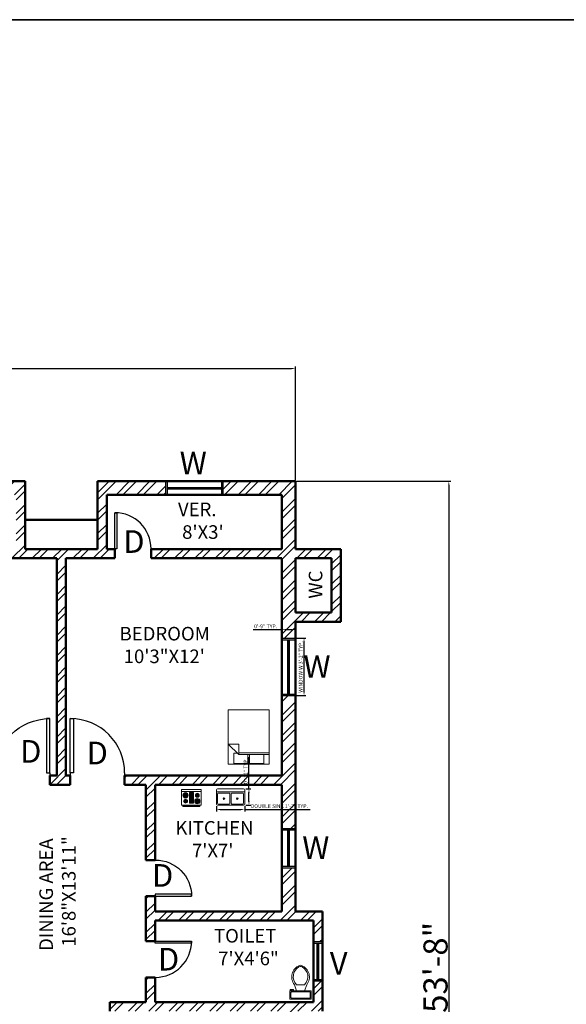
# Model space of a CAD drawing. Units: inches. Extents: x -31485 to -28799, y 18003 to 19130.
# Tile 10 of 15: x -30079 to -29717, y 18478 to 19130. Entities that reach past the tile are written whole.
import ezdxf

# ---------------------------------------------------------------- set-up
doc = ezdxf.new("R2010")
doc.units = ezdxf.units.IN
for name, color, linetype, lineweight in [('A-ANNO-DIMS', 2, 'Continuous', 18), ('A-ANNO-TEXT', 7, 'Continuous', 18), ('A-ANNO-TTLB', 7, 'Continuous', 35), ('A-AREA-IDEN', 7, 'Continuous', 18), ('A-DOOR', 3, 'Continuous', 25), ('A-FLOR-FIXT', 9, 'Continuous', 18), ('A-FURN', 8, 'Continuous', 18), ('A-GLAZ', 4, 'Continuous', 25), ('A-WALL', 7, 'Continuous', 50), ('A-WALL-PATT', 8, 'Continuous', 13)]:
    doc.layers.add(name, color=color, linetype=linetype, lineweight=lineweight)
doc.styles.get("Standard").update_dxf_attribs({"font": 'arial.ttf'})
doc.dimstyles.new('ISO-25', dxfattribs={"dimtxt": 2.5, "dimasz": 2.5, "dimexe": 1.25, "dimexo": 0.625, "dimtad": 1, "dimdec": 0, "dimlunit": 3, "dimtxsty": 'Standard', "dimcen": 2.5, "dimadec": 0, "dimazin": 0, "dimtfac": 1, "dimtdec": 0, "dimtmove": 0, "dimatfit": 3, "dimfxl": 1, "dimarcsym": 0})

# ---------------------------------------------------------------- blocks, each defined once
blk = doc.blocks.new('*U8')
for p, q in [((0, 0), (0, -100)), ((750, 0), (750, -100))]:
    blk.add_line(p, q)
blk.add_lwpolyline([(0, 0), (0, 750), (43.75, 750), (43.75, 0)], close=True)
blk.add_arc((0, 0), 750, 0, 90)
blk = doc.blocks.new('Bed - Queen')
for p, q in [((0, -80.00003), (0, 0)), ((0, 0), (59.99999, 0)), ((59.99999, 0), (59.99999, -80.00003)), ((0, -14.4), (44.8, -14.4)), ((7.99999, -1.2), (28.79998, -1.2)), ((7.99999, -14.4), (7.99999, -1.2)), ((28.79998, -1.2), (28.79998, -14.4)), ((31.19999, -1.2), (51.99999, -1.2)), ((31.19999, -14.4), (31.19999, -1.2)), ((59.99999, -29.6), (44.8, -14.4)), ((44.8, -14.4), (44.8, -29.6)), ((51.99999, -1.2), (51.99999, -16.4)), ((44.8, -16.8), (0, -16.8)), ((51.99999, -16.4), (46.79936, -16.4)), ((44.8, -29.6), (59.99999, -29.6)), ((59.99999, -80.00003), (0, -80.00003))]:
    blk.add_line(p, q)
blk = doc.blocks.new('Range-Oven - 30 in top')
for p, q in [((0, -3), (30, -3)), ((12, -6), (18, -6)), ((13, -20), (13, -6)), ((14, -6), (14, -20)), ((15, -20), (15, -6)), ((16, -6), (16, -20)), ((17, -20), (17, -6)), ((6, -24), (6, -25)), ((8, -25), (8, -24)), ((18, -20), (12, -20)), ((22, -25), (22, -24)), ((24, -24), (24, -25))]:
    blk.add_line(p, q)
for points in [[(0, -24), (0, 0), (30, 0), (30, -24)], [(12, -21), (12, -5), (18, -5), (18, -21)], [(2, -26), (2, -25), (28, -25), (28, -26)]]:
    blk.add_lwpolyline(points, close=True)
for centre, radius in [((6, -9), 4), ((6, -9), 3), ((6, -18), 3), ((6, -9), 2), ((6, -9), 1), ((24, -18), 4), ((24, -9), 3), ((24, -18), 3), ((24, -9), 2), ((24, -9), 1), ((6, -18), 2), ((6, -18), 1), ((24, -18), 2), ((24, -18), 1)]:
    blk.add_circle(centre, radius)
blk = doc.blocks.new('Sink-double - 36 in top')
for p, q in [((-18, -4), (18, -4)), ((-0.75, -18.5), (-0.75, -6.5)), ((0.75, -6.5), (0.75, -18.5))]:
    blk.add_line(p, q)
for points in [[(-16.5, 0), (16.5, 0)], [(-18, -19.5), (-18, -1.5)], [(-16.5, -18.5), (-16.5, -6.5)], [(-15.5, -5.5), (-1.75, -5.5)], [(1.75, -5.5), (15.5, -5.5)], [(16.5, -6.5), (16.5, -18.5)], [(18, -1.5), (18, -19.5)], [(16.5, -21), (-16.5, -21)], [(-1.75, -19.5), (-15.5, -19.5)], [(15.5, -19.5), (1.75, -19.5)]]:
    blk.add_lwpolyline(points)
for centre, radius in [((-8.5, -12.5), 1), ((-8.5, -12.5), 0.5), ((8.5, -12.5), 1), ((8.5, -12.5), 0.5)]:
    blk.add_circle(centre, radius)
for centre, radius, start, end in [((-16.5, -1.5), 1.5, 90, 180), ((16.5, -1.5), 1.5, 0, 90), ((-15.5, -6.5), 1, 90, 180), ((-1.75, -6.5), 1, 0, 90), ((1.75, -6.5), 1, 90, 180), ((15.5, -6.5), 1, 0, 90), ((-16.5, -19.5), 1.5, 180, 270), ((-15.5, -18.5), 1, 180, 270), ((-1.75, -18.5), 1, 270, 0), ((1.75, -18.5), 1, 180, 270), ((15.5, -18.5), 1, 270, 0), ((16.5, -19.5), 1.5, 270, 0)]:
    blk.add_arc(centre, radius, start, end)
blk = doc.blocks.new('Toilet - top')
for p, q in [((-10, -8.5), (-8, -8.5)), ((-10, -9.5), (-10, -8.5)), ((-7, -9.5), (-10, -9.5)), ((-8, -8.5), (-8, -8)), ((-7, -8), (-7, -9.5)), ((-4, -8), (-6, -14)), ((4, -8), (6, -14)), ((9.5, -6), (9.5, -2)), ((4, -14), (-4, -14))]:
    blk.add_line(p, q)
blk.add_lwpolyline([(10.5, -8), (10.5, 0), (-10.5, 0), (-10.5, -8)], close=True)
for points in [[(-9.5, -2), (-9.5, -6)], [(8.5, -1), (-8.5, -1)], [(-8.5, -7), (8.5, -7)]]:
    blk.add_lwpolyline(points)
for centre, radius, start, end in [((-8.62, -1.88), 0.884, 81.8699, 188.1301), ((-8.62, -6.12), 0.884, 171.8699, 278.1301), ((8.62, -1.88), 0.884, 351.8699, 98.1301), ((8.62, -6.12), 0.884, 261.8699, 8.1301), ((3.52, -21.58), 12.17, 141.46911, 247.97143), ((4.2, -21.82), 11.33, 136.36773, 238.94682), ((-3.52, -21.58), 12.17, 292.02843, 38.53071), ((-4.2, -21.82), 11.33, 301.05301, 43.63209), ((0, -27.88), 4, 245.73182, 294.26817), ((0, -29), 4, 254.86053, 285.13947)]:
    blk.add_arc(centre, radius, start, end)
blk = doc.blocks.new('*D188')
at = {"layer": 'A-ANNO-DIMS', "color": 0, "lineweight": -2, "transparency": 16777216}
for p, q in [((-30444.21, 18824.74), (-30444.21, 18900.08)), ((-30441.71, 18898.83), (-29898.71, 18898.83)), ((-29896.21, 18824.74), (-29896.21, 18900.08))]:
    blk.add_line(p, q, dxfattribs=at)
at = {"layer": 'A-ANNO-DIMS', "color": 0, "transparency": 16777216}
for points in [[(-30441.71, 18899.25), (-30441.71, 18898.41), (-30444.21, 18898.83)], [(-29898.71, 18899.25), (-29898.71, 18898.41), (-29896.21, 18898.83)]]:
    blk.add_solid(points, dxfattribs=at)
at = {"layer": 'Defpoints', "color": 0, "transparency": 16777216}
for p in [(-29896.21, 18898.83), (-30444.21, 18824.12), (-29896.21, 18824.12)]:
    blk.add_point(p, dxfattribs=at)
at = {"layer": 'A-ANNO-DIMS', "color": 0, "transparency": 16777216, "insert": (-30170.21, 18907.62), "char_height": 2.5, "attachment_point": 5}
blk.add_mtext('{\\H6.4x;45\'-8"}', dxfattribs=at)
blk = doc.blocks.new('*D189')
at = {"layer": 'A-ANNO-DIMS', "color": 0, "lineweight": -2, "transparency": 16777216}
for p, q in [((-29895.58, 18824.12), (-29793.36, 18824.12)), ((-29794.61, 18821.62), (-29794.61, 18182.62)), ((-29895.58, 18180.12), (-29793.36, 18180.12))]:
    blk.add_line(p, q, dxfattribs=at)
at = {"layer": 'A-ANNO-DIMS', "color": 0, "transparency": 16777216}
for points in [[(-29795.03, 18821.62), (-29794.19, 18821.62), (-29794.61, 18824.12)], [(-29795.03, 18182.62), (-29794.19, 18182.62), (-29794.61, 18180.12)]]:
    blk.add_solid(points, dxfattribs=at)
at = {"layer": 'Defpoints', "color": 0, "transparency": 16777216}
for p in [(-29896.21, 18824.12), (-29896.21, 18180.12), (-29794.61, 18180.12)]:
    blk.add_point(p, dxfattribs=at)
at = {"layer": 'A-ANNO-DIMS', "color": 0, "transparency": 16777216, "insert": (-29803.41, 18502.12), "char_height": 2.5, "attachment_point": 5, "rotation": 90}
blk.add_mtext('{\\H6.4x;53\'-8"}', dxfattribs=at)
blk = doc.blocks.new('WIN-900-W9')
for p, q in [((-29982.21, 18824.12), (-29982.21, 18815.12)), ((-29981.21, 18824.12), (-29981.21, 18815.12)), ((-29981.21, 18820.12), (-29945.21, 18820.12)), ((-29981.21, 18819.62), (-29945.21, 18819.62)), ((-29945.21, 18824.12), (-29945.21, 18815.12)), ((-29944.21, 18824.12), (-29944.21, 18815.12)), ((-29981.21, 18819.12), (-29945.21, 18819.12))]:
    blk.add_line(p, q)
blk = doc.blocks.new('VENT-600-W9')
for p, q in [((-29896.21, 18594.12), (-29905.21, 18594.12)), ((-29896.21, 18593.12), (-29905.21, 18593.12)), ((-29901.21, 18593.12), (-29901.21, 18569.12)), ((-29900.71, 18593.12), (-29900.71, 18569.12)), ((-29900.21, 18593.12), (-29900.21, 18569.12)), ((-29896.21, 18569.12), (-29905.21, 18569.12)), ((-29896.21, 18568.12), (-29905.21, 18568.12))]:
    blk.add_line(p, q)
blk = doc.blocks.new('VENT-600-W6')
for p, q in [((-29884.21, 18519.12), (-29878.21, 18519.12)), ((-29884.21, 18518.12), (-29878.21, 18518.12)), ((-29881.71, 18494.12), (-29881.71, 18518.12)), ((-29881.21, 18494.12), (-29881.21, 18518.12)), ((-29880.71, 18494.12), (-29880.71, 18518.12)), ((-29884.21, 18494.12), (-29878.21, 18494.12)), ((-29884.21, 18493.12), (-29878.21, 18493.12))]:
    blk.add_line(p, q)
blk = doc.blocks.new('*D210')
at = {"layer": 'A-ANNO-DIMS', "color": 0, "lineweight": -2, "transparency": 16777216}
for p, q in [((-29895.58, 18720.12), (-29889.26, 18720.12)), ((-29890.51, 18684.62), (-29890.51, 18717.62)), ((-29895.58, 18682.12), (-29889.26, 18682.12))]:
    blk.add_line(p, q, dxfattribs=at)
at = {"layer": 'A-ANNO-DIMS', "color": 0, "transparency": 16777216}
for points in [[(-29890.92, 18717.62), (-29890.09, 18717.62), (-29890.51, 18720.12)], [(-29890.92, 18684.62), (-29890.09, 18684.62), (-29890.51, 18682.12)]]:
    blk.add_solid(points, dxfattribs=at)
at = {"layer": 'Defpoints', "color": 0, "transparency": 16777216}
for p in [(-29896.21, 18720.12), (-29890.51, 18720.12), (-29896.21, 18682.12)]:
    blk.add_point(p, dxfattribs=at)
at = {"layer": 'A-ANNO-DIMS', "color": 0, "transparency": 16777216, "insert": (-29892.42, 18701.12), "char_height": 2.5, "attachment_point": 5, "rotation": 90}
blk.add_mtext('WINDOW W 3\'-2" TYP.', dxfattribs=at)
blk = doc.blocks.new('*D211')
at = {"layer": 'A-ANNO-DIMS', "color": 0, "lineweight": -2, "transparency": 16777216}
for p, q in [((-29905.21, 18725.82), (-29924.19, 18725.82)), ((-29905.21, 18720.74), (-29905.21, 18727.07)), ((-29898.71, 18725.82), (-29902.71, 18725.82)), ((-29896.21, 18720.74), (-29896.21, 18727.07))]:
    blk.add_line(p, q, dxfattribs=at)
at = {"layer": 'A-ANNO-DIMS', "color": 0, "transparency": 16777216}
for points in [[(-29902.71, 18726.23), (-29902.71, 18725.4), (-29905.21, 18725.82)], [(-29898.71, 18726.23), (-29898.71, 18725.4), (-29896.21, 18725.82)]]:
    blk.add_solid(points, dxfattribs=at)
at = {"layer": 'Defpoints', "color": 0, "transparency": 16777216}
for p in [(-29905.21, 18725.82), (-29905.21, 18720.12), (-29896.21, 18720.12)]:
    blk.add_point(p, dxfattribs=at)
at = {"layer": 'A-ANNO-DIMS', "color": 0, "transparency": 16777216, "insert": (-29915.95, 18727.72), "char_height": 2.5, "attachment_point": 5}
blk.add_mtext('0\'-9" TYP.', dxfattribs=at)
blk = doc.blocks.new('*D252')
at = {"layer": 'A-ANNO-DIMS', "color": 0, "lineweight": -2, "transparency": 16777216}
for p, q in [((-29948.54, 18608.87), (-29948.54, 18605.43)), ((-29946.04, 18606.68), (-29932.29, 18606.68)), ((-29929.79, 18608.87), (-29929.79, 18605.43)), ((-29929.79, 18606.68), (-29886.47, 18606.68))]:
    blk.add_line(p, q, dxfattribs=at)
at = {"layer": 'A-ANNO-DIMS', "color": 0, "transparency": 16777216}
for points in [[(-29946.04, 18607.1), (-29946.04, 18606.26), (-29948.54, 18606.68)], [(-29932.29, 18607.1), (-29932.29, 18606.26), (-29929.79, 18606.68)]]:
    blk.add_solid(points, dxfattribs=at)
at = {"layer": 'Defpoints', "color": 0, "transparency": 16777216}
for p in [(-29948.54, 18609.49), (-29929.79, 18609.49), (-29929.79, 18606.68)]:
    blk.add_point(p, dxfattribs=at)
at = {"layer": 'A-ANNO-DIMS', "color": 0, "transparency": 16777216, "insert": (-29906.88, 18608.6), "char_height": 2.5, "attachment_point": 5}
blk.add_mtext('DOUBLE SINK 1\'-7" TYP.', dxfattribs=at)
blk = doc.blocks.new('*D253')
at = {"layer": 'A-ANNO-DIMS', "color": 0, "lineweight": -2, "transparency": 16777216}
for p, q in [((-29926.97, 18620.43), (-29926.97, 18641.36)), ((-29929.16, 18620.43), (-29925.72, 18620.43)), ((-29926.97, 18611.99), (-29926.97, 18617.93)), ((-29929.16, 18609.49), (-29925.72, 18609.49))]:
    blk.add_line(p, q, dxfattribs=at)
at = {"layer": 'A-ANNO-DIMS', "color": 0, "transparency": 16777216}
for points in [[(-29927.39, 18617.93), (-29926.56, 18617.93), (-29926.97, 18620.43)], [(-29927.39, 18611.99), (-29926.56, 18611.99), (-29926.97, 18609.49)]]:
    blk.add_solid(points, dxfattribs=at)
at = {"layer": 'Defpoints', "color": 0, "transparency": 16777216}
for p in [(-29929.79, 18620.43), (-29926.97, 18620.43), (-29929.79, 18609.49)]:
    blk.add_point(p, dxfattribs=at)
at = {"layer": 'A-ANNO-DIMS', "color": 0, "transparency": 16777216, "insert": (-29928.87, 18632.15), "char_height": 2.5, "attachment_point": 5, "rotation": 90}
blk.add_mtext('0\'-11" TYP.', dxfattribs=at)

msp = doc.modelspace()

# ---------------------------------------------------------------- hatches: boundary and pattern name
at = {"layer": 'A-WALL-PATT'}
h = msp.add_hatch(dxfattribs=at)
h.set_pattern_fill('ANSI32', color=256)
h.paths.add_polyline_path([(-30435.21, 18779.12), (-30435.21, 18815.12), (-30406.21, 18815.12), (-30406.21, 18824.12), (-30444.21, 18824.12), (-30444.21, 18779.12), (-30474.21, 18779.12), (-30474.21, 18731.12), (-30444.21, 18731.12), (-30444.21, 18704.18), (-30435.21, 18704.18), (-30435.21, 18773.12), (-30369.28, 18773.12), (-30369.28, 18779.12)])
h.paths.add_polyline_path([(-30444.21, 18773.12), (-30444.21, 18737.12), (-30468.21, 18737.12), (-30468.21, 18773.12)], flags=16)
h.paths.add_polyline_path([(-30333.21, 18824.12), (-30368.21, 18824.12), (-30368.21, 18815.12), (-30339.21, 18815.12), (-30339.21, 18779.12), (-30345.28, 18779.12), (-30345.28, 18773.12), (-30312.21, 18773.12), (-30312.21, 18629.12), (-30315.41, 18629.12), (-30315.41, 18626.12), (-30315.41, 18623.12), (-30299.19, 18623.12), (-30299.19, 18629.12), (-30306.21, 18629.12), (-30306.21, 18773.12), (-30274.83, 18773.12), (-30274.83, 18779.12), (-30279.21, 18779.12), (-30279.21, 18815.12), (-30250.21, 18815.12), (-30250.21, 18824.12), (-30285.21, 18824.12), (-30285.21, 18779.12), (-30333.21, 18779.12)])
h.paths.add_polyline_path([(-30177.21, 18779.12), (-30177.21, 18815.12), (-30148.21, 18815.12), (-30148.21, 18824.12), (-30212.21, 18824.12), (-30212.21, 18815.12), (-30183.21, 18815.12), (-30183.21, 18779.12), (-30250.83, 18779.12), (-30250.83, 18776.12), (-30250.83, 18773.12), (-30183.21, 18773.12), (-30183.21, 18720.12), (-30177.21, 18720.12), (-30177.21, 18773.12), (-30110.84, 18773.12), (-30110.84, 18779.12)])
h.paths.add_polyline_path([(-30015.86, 18779.12), (-30021.21, 18779.12), (-30021.21, 18815.12), (-29982.21, 18815.12), (-29982.21, 18824.12), (-30027.21, 18824.12), (-30027.21, 18779.12), (-30075.21, 18779.12), (-30075.21, 18824.12), (-30110.21, 18824.12), (-30110.21, 18815.12), (-30081.21, 18815.12), (-30081.21, 18779.12), (-30086.84, 18779.12), (-30086.84, 18776.12), (-30086.84, 18773.12), (-30054.21, 18773.12), (-30054.21, 18629.12), (-30058.98, 18629.12), (-30058.98, 18623.12), (-30045.32, 18623.12), (-30045.32, 18629.12), (-30048.21, 18629.12), (-30048.21, 18773.12), (-30015.86, 18773.12)])
h.paths.add_polyline_path([(-29866.21, 18779.12), (-29896.21, 18779.12), (-29896.21, 18824.12), (-29944.21, 18824.12), (-29944.21, 18815.12), (-29905.21, 18815.12), (-29905.21, 18779.12), (-29991.86, 18779.12), (-29991.86, 18776.12), (-29991.86, 18773.12), (-29905.21, 18773.12), (-29905.21, 18720.12), (-29896.21, 18720.12), (-29896.21, 18731.12), (-29866.21, 18731.12)])
h.paths.add_polyline_path([(-29896.21, 18773.12), (-29872.21, 18773.12), (-29872.21, 18737.12), (-29896.21, 18737.12)], flags=16)
h.paths.add_polyline_path([(-29896.21, 18682.12), (-29905.21, 18682.12), (-29905.21, 18629.12), (-30009.32, 18629.12), (-30009.32, 18626.12), (-30009.32, 18623.12), (-29995.21, 18623.12), (-29995.21, 18573.22), (-29989.21, 18573.22), (-29989.21, 18623.12), (-29905.21, 18623.12), (-29905.21, 18594.12), (-29896.21, 18594.12)])
h.paths.add_polyline_path([(-30094.98, 18629.12), (-30177.21, 18629.12), (-30177.21, 18682.12), (-30183.21, 18682.12), (-30183.21, 18629.12), (-30263.19, 18629.12), (-30263.19, 18626.12), (-30263.19, 18623.12), (-30183.21, 18623.12), (-30183.21, 18425.12), (-30234.21, 18425.12), (-30234.21, 18408.38), (-30228.21, 18408.38), (-30228.21, 18419.12), (-30112.21, 18419.12), (-30112.21, 18406.94), (-30106.21, 18406.94), (-30106.21, 18425.12), (-30177.21, 18425.12), (-30177.21, 18623.12), (-30094.98, 18623.12)])
h.paths.add_polyline_path([(-29896.21, 18568.12), (-29905.21, 18568.12), (-29905.21, 18539.12), (-29989.21, 18539.12), (-29989.21, 18549.22), (-29992.21, 18549.22), (-29995.21, 18549.22), (-29995.21, 18519.45), (-29989.21, 18519.45), (-29989.21, 18533.12), (-29884.21, 18533.12), (-29884.21, 18519.12), (-29878.21, 18519.12), (-29878.21, 18539.12), (-29896.21, 18539.12)])
h.paths.add_polyline_path([(-29878.21, 18493.12), (-29884.21, 18493.12), (-29884.21, 18479.12), (-29989.21, 18479.12), (-29989.21, 18495.45), (-29992.21, 18495.45), (-29995.21, 18495.45), (-29995.21, 18479.12), (-30019.21, 18479.12), (-30019.21, 18473.12), (-29905.21, 18473.12), (-29905.21, 18438.12), (-29896.21, 18438.12), (-29896.21, 18473.12), (-29878.21, 18473.12)])
h.paths.add_polyline_path([(-29896.21, 18400.12), (-29905.21, 18400.12), (-29905.21, 18365.12), (-29952.21, 18365.12), (-29952.21, 18359.12), (-29905.21, 18359.12), (-29905.21, 18309.79), (-29896.21, 18309.79), (-29896.21, 18317.12), (-29866.21, 18317.12), (-29866.21, 18365.12), (-29896.21, 18365.12)])
h.paths.add_polyline_path([(-29896.21, 18359.12), (-29872.21, 18359.12), (-29872.21, 18323.12), (-29896.21, 18323.12)], flags=16)
h.paths.add_polyline_path([(-29990.21, 18365.12), (-30043.21, 18365.12), (-30050.35, 18365.12), (-30050.35, 18359.12), (-29990.21, 18359.12)])
h.paths.add_polyline_path([(-29896.21, 18271.79), (-29905.21, 18271.79), (-29905.21, 18243.12), (-30046.21, 18243.12), (-30046.21, 18315.12), (-30055.46, 18315.12), (-30055.46, 18309.12), (-30052.21, 18309.12), (-30052.21, 18219.12), (-30066.21, 18219.12), (-30066.21, 18213.12), (-30052.21, 18213.12), (-30052.21, 18180.12), (-29993.21, 18180.12), (-29993.21, 18189.12), (-30046.21, 18189.12), (-30046.21, 18237.12), (-29905.21, 18237.12), (-29905.21, 18189.12), (-29955.21, 18189.12), (-29955.21, 18180.12), (-29896.21, 18180.12)])
h.paths.add_polyline_path([(-30092.21, 18219.12), (-30106.21, 18219.12), (-30106.21, 18309.12), (-30079.46, 18309.12), (-30079.46, 18315.12), (-30106.21, 18315.12), (-30106.21, 18359.12), (-30086.35, 18359.12), (-30086.35, 18365.12), (-30106.21, 18365.12), (-30106.21, 18370.94), (-30112.21, 18370.94), (-30112.21, 18189.12), (-30151.21, 18189.12), (-30151.21, 18180.12), (-30106.21, 18180.12), (-30106.21, 18213.12), (-30092.21, 18213.12)])
h.paths.add_polyline_path([(-30189.21, 18189.12), (-30228.21, 18189.12), (-30228.21, 18225.12), (-30234.21, 18225.12), (-30234.21, 18219.12), (-30248.21, 18219.12), (-30248.21, 18213.12), (-30234.21, 18213.12), (-30234.21, 18180.12), (-30189.21, 18180.12)])
h.paths.add_polyline_path([(-30288.21, 18213.12), (-30274.21, 18213.12), (-30274.21, 18219.12), (-30288.21, 18219.12), (-30288.21, 18309.12), (-30285.87, 18309.12), (-30285.87, 18315.12), (-30294.21, 18315.12), (-30294.21, 18243.12), (-30435.21, 18243.12), (-30435.21, 18263.9), (-30444.21, 18263.9), (-30444.21, 18180.12), (-30383.71, 18180.12), (-30383.71, 18189.12), (-30435.21, 18189.12), (-30435.21, 18237.12), (-30294.21, 18237.12), (-30294.21, 18189.12), (-30345.71, 18189.12), (-30345.71, 18180.12), (-30288.21, 18180.12)])
h.paths.add_polyline_path([(-30435.21, 18359.12), (-30388.21, 18359.12), (-30388.21, 18365.12), (-30435.21, 18365.12), (-30435.21, 18400.12), (-30444.21, 18400.12), (-30444.21, 18365.12), (-30474.21, 18365.12), (-30474.21, 18317.12), (-30444.21, 18317.12), (-30444.21, 18301.9), (-30435.21, 18301.9)])
h.paths.add_polyline_path([(-30444.21, 18323.12), (-30468.21, 18323.12), (-30468.21, 18359.12), (-30444.21, 18359.12)], flags=16)
h.paths.add_polyline_path([(-30294.54, 18365.12), (-30297.21, 18365.12), (-30350.21, 18365.12), (-30350.21, 18359.12), (-30294.54, 18359.12)])
h.paths.add_polyline_path([(-30228.21, 18372.38), (-30234.21, 18372.38), (-30234.21, 18365.12), (-30258.54, 18365.12), (-30258.54, 18359.12), (-30234.21, 18359.12), (-30234.21, 18315.12), (-30261.87, 18315.12), (-30261.87, 18309.12), (-30234.21, 18309.12), (-30234.21, 18225.12), (-30228.21, 18225.12)])
h.paths.add_polyline_path([(-30375.49, 18525.25), (-30375.54, 18525.25), (-30375.54, 18526.65), (-30351.51, 18526.65), (-30351.51, 18525.25), (-30375.49, 18525.25, 0.400923), (-30351.21, 18502.63), (-30351.21, 18502.64), (-30345.21, 18502.64), (-30345.21, 18479.12), (-30325.98, 18479.12), (-30325.98, 18473.12), (-30435.21, 18473.12), (-30435.21, 18437.12), (-30439.21, 18437.12), (-30439.21, 18401.12), (-30440.21, 18401.12), (-30440.21, 18437.12), (-30444.21, 18437.12), (-30444.21, 18473.12), (-30462.21, 18473.12), (-30462.21, 18494.12), (-30456.21, 18494.12), (-30456.21, 18479.12), (-30351.21, 18479.12), (-30351.21, 18502.63), (-30351.51, 18502.63, -0.39722)])
h.paths.add_polyline_path([(-30345.21, 18556.53), (-30351.21, 18556.53), (-30351.21, 18539.12), (-30435.21, 18539.12), (-30435.21, 18568.12), (-30444.21, 18568.12), (-30444.21, 18539.12), (-30462.21, 18539.12), (-30462.21, 18519.12), (-30456.21, 18519.12), (-30456.21, 18533.12), (-30351.21, 18533.12), (-30351.21, 18526.64), (-30345.21, 18526.64)])
h.paths.add_polyline_path([(-30344.41, 18629.12), (-30435.21, 18629.12), (-30435.21, 18666.18), (-30444.21, 18666.18), (-30444.21, 18594.12), (-30435.21, 18594.12), (-30435.21, 18623.12), (-30351.21, 18623.12), (-30351.21, 18580.56), (-30347.87, 18580.56), (-30345.21, 18580.53), (-30345.21, 18623.12)])

# ---------------------------------------------------------------- linework, layer by layer
at = {"layer": 'A-ANNO-TTLB'}
msp.add_lwpolyline([(-31485.1, 19129.94), (-28798.64, 19129.94), (-28798.64, 18002.86), (-31485.1, 18002.86)], close=True, dxfattribs=at)
at = {"layer": 'A-WALL'}
for p, q in [((-30285.21, 18824.12), (-30075.21, 18824.12)), ((-30075.21, 18779.12), (-30075.21, 18824.12)), ((-30027.21, 18779.12), (-30027.21, 18824.12)), ((-30027.21, 18824.12), (-29896.21, 18824.12)), ((-29896.21, 18824.12), (-29896.21, 18779.12)), ((-30021.21, 18779.12), (-30021.21, 18815.12)), ((-30021.21, 18815.12), (-29905.21, 18815.12)), ((-29905.21, 18815.12), (-29905.21, 18779.12)), ((-30075.21, 18798.62), (-30027.21, 18798.62)), ((-30075.21, 18779.12), (-30027.21, 18779.12)), ((-30021.21, 18779.12), (-30015.86, 18779.12)), ((-30015.86, 18779.12), (-30015.86, 18773.12)), ((-29991.86, 18779.12), (-29991.86, 18773.12)), ((-29991.86, 18779.12), (-29905.21, 18779.12)), ((-29896.21, 18779.12), (-29866.21, 18779.12)), ((-29866.21, 18779.12), (-29866.21, 18731.12)), ((-30086.84, 18773.12), (-30054.21, 18773.12)), ((-30054.21, 18629.12), (-30054.21, 18773.12)), ((-30048.21, 18629.12), (-30048.21, 18773.12)), ((-30048.21, 18773.12), (-30015.86, 18773.12)), ((-29991.86, 18773.12), (-29905.21, 18773.12)), ((-29905.21, 18773.12), (-29905.21, 18629.12)), ((-29896.21, 18773.12), (-29872.21, 18773.12)), ((-29896.21, 18773.12), (-29896.21, 18737.12)), ((-29872.21, 18773.12), (-29872.21, 18737.12)), ((-29896.21, 18737.12), (-29872.21, 18737.12)), ((-29896.21, 18731.12), (-29866.21, 18731.12)), ((-29896.21, 18731.12), (-29896.21, 18539.12)), ((-30058.98, 18629.12), (-30058.98, 18623.12)), ((-30058.98, 18629.12), (-30054.21, 18629.12)), ((-30048.21, 18629.12), (-30045.32, 18629.12)), ((-30045.32, 18629.12), (-30045.32, 18623.12)), ((-30009.32, 18629.12), (-30009.32, 18623.12)), ((-30009.32, 18629.12), (-29905.21, 18629.12)), ((-30058.98, 18623.12), (-30045.32, 18623.12)), ((-30009.32, 18623.12), (-29995.21, 18623.12)), ((-29995.21, 18623.12), (-29995.21, 18573.22)), ((-29989.21, 18623.12), (-29989.21, 18573.22)), ((-29989.21, 18623.12), (-29905.21, 18623.12)), ((-29905.21, 18623.12), (-29905.21, 18539.12)), ((-29995.21, 18573.22), (-29989.21, 18573.22)), ((-29995.21, 18549.22), (-29989.21, 18549.22)), ((-29995.21, 18549.22), (-29995.21, 18519.45)), ((-29989.21, 18549.22), (-29989.21, 18539.12)), ((-29989.21, 18539.12), (-29905.21, 18539.12)), ((-29896.21, 18539.12), (-29878.21, 18539.12)), ((-29878.21, 18539.12), (-29878.21, 18473.12)), ((-29989.21, 18533.12), (-29884.21, 18533.12)), ((-29989.21, 18533.12), (-29989.21, 18519.45)), ((-29884.21, 18533.12), (-29884.21, 18479.12)), ((-29995.21, 18519.45), (-29989.21, 18519.45)), ((-29995.21, 18495.45), (-29989.21, 18495.45)), ((-29995.21, 18495.45), (-29995.21, 18479.12)), ((-29989.21, 18495.45), (-29989.21, 18479.12)), ((-30019.21, 18479.12), (-29995.21, 18479.12)), ((-30019.21, 18479.12), (-30019.21, 18473.12)), ((-29989.21, 18479.12), (-29884.21, 18479.12))]:
    msp.add_line(p, q, dxfattribs=at)

# ---------------------------------------------------------------- block references
at = {"layer": 'A-DOOR'}
for p, xscale, yscale, zscale in [((-30015.86, 18779.32), 0.0320000000000051, 0.0320000000000051, 0.0320000000000051), ((-30058.98, 18630.92), -0.0479999003599065, 0.0479999003599065, 0.0479999003599065), ((-30045.32, 18630.92), 0.0479999999999911, 0.0479999999999911, 0.0479999999999911)]:
    msp.add_blockref('*U8', p, dxfattribs=dict(at, xscale=xscale, yscale=yscale, zscale=zscale))
at = {"layer": 'A-DOOR', "rotation": 270}
for p, xscale, yscale, zscale in [((-29989.01, 18549.22), -0.0320000000000009, 0.0320000000000009, 0.0320000000000009), ((-29989.01, 18519.45), 0.0320000112062311, 0.0320000112062311, 0.0320000112062311)]:
    msp.add_blockref('*U8', p, dxfattribs=dict(at, xscale=xscale, yscale=yscale, zscale=zscale))
at = {"layer": 'A-FLOR-FIXT'}
for name, p, xscale, yscale, zscale in [('Range-Oven - 30 in top', (-29971.59, 18620.01), 0.4333333333333334, 0.4333333333333334, 0.4333333333333334), ('Sink-double - 36 in top', (-29939.16, 18620.43), 0.5208333333333334, 0.5208333333333334, 0.5208333333333334)]:
    msp.add_blockref(name, p, dxfattribs=dict(at, xscale=xscale, yscale=yscale, zscale=zscale))
at = {"layer": 'A-FLOR-FIXT', "xscale": -0.6786300354967684, "yscale": 0.6786300354967684, "zscale": 0.6786300354967684, "rotation": 180}
msp.add_blockref('Toilet - top', (-29892.81, 18481.08), dxfattribs=at)
at = {"layer": 'A-FURN', "xscale": 0.4514551267732207, "yscale": 0.4514551267732207, "zscale": 0.4514551267732207, "rotation": 180}
msp.add_blockref('Bed - Queen', (-29913.56, 18636.64), dxfattribs=at)
at = {"layer": 'A-GLAZ'}
for name in ['WIN-900-W9', 'VENT-600-W6']:
    msp.add_blockref(name, (0, 0), dxfattribs=at)
for name, p, rotation in [('WIN-900-W9', (-11081.09, 48664.32), 90.00000000001586), ('VENT-600-W9', (-59801.41, 37162.23), 180)]:
    msp.add_blockref(name, p, dxfattribs=dict(at, rotation=rotation))

# ---------------------------------------------------------------- texts
at = {"layer": 'A-ANNO-TEXT', "char_height": 15, "attachment_point": 1}
for s, insert in [('{W}', (-29972.88, 18843.7)), ('{D}', (-30010.21, 18791.7)), ('{W}', (-29890.9, 18708.92)), ('{D}', (-30078.52, 18652.69)), ('{D}', (-30034.53, 18651.6)), ('{W}', (-29891.7, 18588.95)), ('{D}', (-29991.19, 18570.49)), ('{D}', (-29987.29, 18515)), ('{V}', (-29873.45, 18512.32))]:
    msp.add_mtext_dynamic_manual_height_columns(s, width=1155.9407, gutter_width=12.5, heights=[0], dxfattribs=dict(at, insert=insert))
at = {"layer": 'A-AREA-IDEN', "char_height": 9, "attachment_point": 1}
for s, insert in [("{    VER.\\P     8'X3'}", (-29984.99, 18810.01)), ('{BEDROOM\\P 10\'3"X12\'}', (-30012.68, 18727.67)), ("{ KITCHEN\\P     7'X7'}", (-29978.48, 18599.01)), ('{   TOILET\\P    7\'X4\'6"}', (-29958.37, 18527.52))]:
    msp.add_mtext_dynamic_manual_height_columns(s, width=1354.6859, gutter_width=12.5, heights=[0], dxfattribs=dict(at, insert=insert))
at = {"layer": 'A-AREA-IDEN', "char_height": 9, "attachment_point": 1, "rotation": 90}
for s, insert in [('{WC}', (-29887.38, 18746.39)), ('{ DINING AREA\\P  16\'8"X13\'11"}', (-30065.81, 18510.26))]:
    msp.add_mtext_dynamic_manual_height_columns(s, width=1354.6859, gutter_width=12.5, heights=[0], dxfattribs=dict(at, insert=insert))

# ---------------------------------------------------------------- dimensions: what is measured, and where the dimension line sits
at = {"layer": 'A-ANNO-DIMS'}
for base, p1, p2, text, override, picture, middle in [((-29896.21, 18898.83), (-30444.21, 18824.12), (-29896.21, 18824.12), '{\\H6.4x;<>}', {"dimclrd": 0, "dimclre": 0, "dimclrt": 0}, '*D188', (-30170.21, 18907.62)), ((-29929.7852914, 18606.68106605), (-29948.5352914, 18609.49356605), (-29929.7852914, 18609.49356605), 'DOUBLE SINK <> TYP.', {"dimdec": 1, "dimlfac": 1, "dimrnd": 0, "dimzin": 1, "dimdsep": 46, "dimlunit": 4, "dimfrac": 2}, '*D252', (-29906.87601446, 18608.59955173))]:
    dim = msp.add_linear_dim(base=base, p1=p1, p2=p2, text=text, dimstyle='ISO-25', override=override, dxfattribs=at)
    dim.commit()
    dim.dimension.update_dxf_attribs({"geometry": picture, "text_midpoint": middle})
for base, p1, p2, angle, text, override, picture, middle in [((-29794.61, 18180.12), (-29896.21, 18824.12), (-29896.21, 18180.12), 90, '{\\H6.4x;<>}', {"dimclrd": 0, "dimclre": 0, "dimclrt": 0}, '*D189', (-29803.41, 18502.12)), ((-29905.21, 18725.82), (-29896.21, 18720.12), (-29905.21, 18720.12), 180, '<> TYP.', {"dimdec": 1, "dimlfac": 1, "dimrnd": 0, "dimzin": 1, "dimdsep": 46, "dimlunit": 4, "dimfrac": 2}, '*D211', (-29915.95, 18727.72)), ((-29890.51, 18720.12), (-29896.21, 18682.12), (-29896.21, 18720.12), 90, 'WINDOW W <> TYP.', {"dimdec": 1, "dimlfac": 1, "dimrnd": 0, "dimzin": 1, "dimdsep": 46, "dimlunit": 4, "dimfrac": 2}, '*D210', (-29892.42, 18701.12)), ((-29926.97, 18620.43), (-29929.79, 18609.49), (-29929.79, 18620.43), 90, '<> TYP.', {"dimdec": 1, "dimlfac": 1, "dimrnd": 0, "dimzin": 1, "dimdsep": 46, "dimlunit": 4, "dimfrac": 2}, '*D253', (-29928.87, 18632.15))]:
    dim = msp.add_linear_dim(base=base, p1=p1, p2=p2, angle=angle, text=text, dimstyle='ISO-25', override=override, dxfattribs=at)
    dim.commit()
    dim.dimension.update_dxf_attribs({"geometry": picture, "text_midpoint": middle})

doc.saveas('drawing.dxf')
